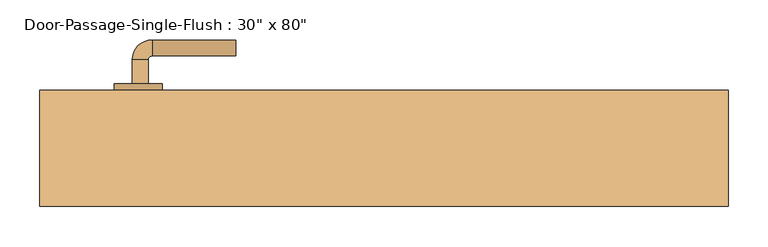
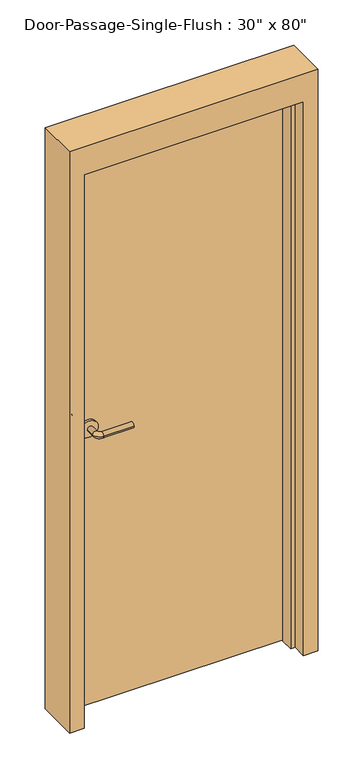
"""IFC4 building model written with IfcOpenShell, lengths in millimetres: door geometry."""

from ifc_helpers import new_model, si_unit, point, frame, frame_2d, origin, origin_with_axes, place, context, project, spatial, polyline, circle_curve, ellipse_curve, trimmed, segment, composite_curve, outline, extrude, faceted_brep, source, transform, mapped, element, save
from ifc_brep_helpers import plane_surface, cylinder_surface, revolved_surface, advanced_brep


def door_bb4af967(model_context):
    return source(origin(), model_context, "Body", "SolidModel", [
        advanced_brep(
        [(-315.990625, 4.7, 1016.0), (-295.990625, 4.7, 1016.0), (-295.990625, -25.3, 1016.0), (-315.990625, -25.3, 1016.0), (-290.990625, -30.3, 1016.0), (-290.990625, -50.3, 1016.0), (-185.990625, -50.3, 1016.0), (-185.990625, -30.3, 1016.0)],
        [
            (0, 1, circle_curve(frame((-305.990625, 4.7, 1016.0), z_axis=(0.0, 1.0, 0.0), x_axis=(1.0, 0.0, 0.0)), 10.0)),
            (1, 0, circle_curve(frame((-305.990625, 4.7, 1016.0), z_axis=(0.0, 1.0, 0.0), x_axis=(1.0, 0.0, 0.0)), 10.0)),
            (1, 2),
            (2, 3, circle_curve(frame((-305.990625, -25.3, 1016.0), z_axis=(0.0, 1.0, 0.0), x_axis=(1.0, 0.0, 0.0)), 10.0)),
            (3, 0),
            (3, 2, circle_curve(frame((-305.990625, -25.3, 1016.0), z_axis=(0.0, 1.0, 0.0), x_axis=(1.0, 0.0, 0.0)), 10.0)),
            (4, 5, circle_curve(frame((-290.990625, -40.3, 1016.0), z_axis=(-1.0, 0.0, 0.0), x_axis=(0.0, 1.0, 0.0)), 10.0)),
            (5, 3, circle_curve(frame((-290.990625, -25.3, 1016.0), z_axis=(0.0, 0.0, -1.0), x_axis=(-1.0, 0.0, 0.0)), 25.0)),
            (2, 4, circle_curve(frame((-290.990625, -25.3, 1016.0), z_axis=(0.0, 0.0, 1.0), x_axis=(-1.0, 0.0, 0.0)), 5.0)),
            (5, 4, circle_curve(frame((-290.990625, -40.3, 1016.0), z_axis=(-1.0, 0.0, 0.0), x_axis=(0.0, 1.0, 0.0)), 10.0)),
            (6, 7, circle_curve(frame((-185.990625, -40.3, 1016.0), z_axis=(1.0, 0.0, 0.0), x_axis=(0.0, 1.0, 0.0)), 10.0)),
            (7, 6, circle_curve(frame((-185.990625, -40.3, 1016.0), z_axis=(1.0, 0.0, 0.0), x_axis=(0.0, 1.0, 0.0)), 10.0)),
            (4, 7),
            (6, 5),
        ],
        [
            plane_surface(frame((-305.990625, 4.7, 1016.0), z_axis=(0.0, 1.0, 0.0), x_axis=(0.0, 0.0, 1.0))),
            cylinder_surface(frame((-305.990625, 4.7, 1016.0), z_axis=(0.0, 1.0, 0.0), x_axis=(1.0, 0.0, 0.0)), 10.0),
            revolved_surface(trimmed(ellipse_curve(frame((-305.990625, -25.3, 1016.0), z_axis=(0.0, -1.0, 0.0), x_axis=(1.0, 0.0, 0.0)), 10.0, 10.0), [point((-315.990625, -25.3, 1016.0))], [point((-295.990625, -25.3, 1016.0))], True, "CARTESIAN"), (-290.990625, -25.3, 1016.0), (0.0, 0.0, -1.0)),
            revolved_surface(trimmed(ellipse_curve(frame((-305.990625, -25.3, 1016.0), z_axis=(0.0, -1.0, 0.0), x_axis=(1.0, 0.0, 0.0)), 10.0, 10.0), [point((-295.990625, -25.3, 1016.0))], [point((-315.990625, -25.3, 1016.0))], True, "CARTESIAN"), (-290.990625, -25.3, 1016.0), (0.0, 0.0, -1.0)),
            plane_surface(frame((-185.990625, -40.3, 1016.0), z_axis=(1.0, 0.0, 0.0), x_axis=(0.0, 0.0, 1.0))),
            cylinder_surface(frame((-290.990625, -40.3, 1016.0), z_axis=(-1.0, 0.0, 0.0), x_axis=(0.0, 1.0, 0.0)), 10.0),
        ],
        [
            (0, [[1, 2]]),
            (1, [[3, 4, 5, -2]]),
            (1, [[-5, 6, -3, -1]]),
            (2, [[7, 8, -4, 9]]),
            (3, [[10, -9, -6, -8]]),
            (4, [[11, 12]]),
            (5, [[13, -11, 14, -7]]),
            (5, [[-14, -12, -13, -10]]),
        ],
    ),
        extrude(outline(composite_curve([segment(trimmed(circle_curve(frame_2d((1016.0, -308.490625)), 30.0), [point((1016.0, -338.490625))], [point((1016.0, -278.490625))], False, "CARTESIAN"), True, "CONTINUOUS"), segment(trimmed(circle_curve(frame_2d((1016.0, -308.490625)), 30.0), [point((1016.0, -278.490625))], [point((1016.0, -338.490625))], False, "CARTESIAN"), True, "CONTINUOUS")], self_intersect=False)), frame((0.0, 4.7, 0.0), z_axis=(0.0, 1.0, 0.0), x_axis=(0.0, 0.0, 1.0)), (0.0, 0.0, 1.0), 8.0),
        advanced_brep(
        [(-315.990625, 65.15, 1016.0), (-295.990625, 65.15, 1016.0), (-315.990625, 95.15, 1016.0), (-295.990625, 95.15, 1016.0), (-290.990625, 100.15, 1016.0), (-290.990625, 120.15, 1016.0), (-185.990625, 120.15, 1016.0), (-185.990625, 100.15, 1016.0)],
        [
            (0, 1, circle_curve(frame((-305.990625, 65.15, 1016.0), z_axis=(0.0, -1.0, 0.0), x_axis=(1.0, 0.0, 0.0)), 10.0)),
            (1, 0, circle_curve(frame((-305.990625, 65.15, 1016.0), z_axis=(0.0, -1.0, 0.0), x_axis=(1.0, 0.0, 0.0)), 10.0)),
            (0, 2),
            (2, 3, circle_curve(frame((-305.990625, 95.15, 1016.0), z_axis=(0.0, -1.0, 0.0), x_axis=(1.0, 0.0, 0.0)), 10.0)),
            (3, 1),
            (3, 2, circle_curve(frame((-305.990625, 95.15, 1016.0), z_axis=(0.0, -1.0, 0.0), x_axis=(1.0, 0.0, 0.0)), 10.0)),
            (4, 3, circle_curve(frame((-290.990625, 95.15, 1016.0), z_axis=(0.0, 0.0, 1.0), x_axis=(-1.0, 0.0, 0.0)), 5.0)),
            (2, 5, circle_curve(frame((-290.990625, 95.15, 1016.0), z_axis=(0.0, 0.0, -1.0), x_axis=(-1.0, 0.0, 0.0)), 25.0)),
            (5, 4, circle_curve(frame((-290.990625, 110.15, 1016.0), z_axis=(-1.0, 0.0, 0.0), x_axis=(0.0, -1.0, 0.0)), 10.0)),
            (4, 5, circle_curve(frame((-290.990625, 110.15, 1016.0), z_axis=(-1.0, 0.0, 0.0), x_axis=(0.0, -1.0, 0.0)), 10.0)),
            (6, 7, circle_curve(frame((-185.990625, 110.15, 1016.0), z_axis=(1.0, 0.0, 0.0), x_axis=(0.0, -1.0, 0.0)), 10.0)),
            (7, 6, circle_curve(frame((-185.990625, 110.15, 1016.0), z_axis=(1.0, 0.0, 0.0), x_axis=(0.0, -1.0, 0.0)), 10.0)),
            (5, 6),
            (7, 4),
        ],
        [
            plane_surface(frame((-305.990625, 65.15, 1016.0), z_axis=(0.0, -1.0, 0.0), x_axis=(0.0, 0.0, 1.0))),
            cylinder_surface(frame((-305.990625, 65.15, 1016.0), z_axis=(0.0, -1.0, 0.0), x_axis=(1.0, 0.0, 0.0)), 10.0),
            revolved_surface(trimmed(ellipse_curve(frame((-305.990625, 95.15, 1016.0), z_axis=(0.0, -1.0, 0.0), x_axis=(1.0, 0.0, 0.0)), 10.0, 10.0), [point((-315.990625, 95.15, 1016.0))], [point((-295.990625, 95.15, 1016.0))], True, "CARTESIAN"), (-290.990625, 95.15, 1016.0), (0.0, 0.0, -1.0)),
            revolved_surface(trimmed(ellipse_curve(frame((-305.990625, 95.15, 1016.0), z_axis=(0.0, -1.0, 0.0), x_axis=(1.0, 0.0, 0.0)), 10.0, 10.0), [point((-295.990625, 95.15, 1016.0))], [point((-315.990625, 95.15, 1016.0))], True, "CARTESIAN"), (-290.990625, 95.15, 1016.0), (0.0, 0.0, -1.0)),
            plane_surface(frame((-185.990625, 110.15, 1016.0), z_axis=(1.0, 0.0, 0.0), x_axis=(0.0, 0.0, 1.0))),
            cylinder_surface(frame((-290.990625, 110.15, 1016.0), z_axis=(-1.0, 0.0, 0.0), x_axis=(0.0, -1.0, 0.0)), 10.0),
        ],
        [
            (0, [[1, 2]]),
            (1, [[-1, 3, 4, 5]]),
            (1, [[-2, -5, 6, -3]]),
            (2, [[7, -4, 8, 9]]),
            (3, [[-8, -6, -7, 10]]),
            (4, [[11, 12]]),
            (5, [[-9, 13, -12, 14]]),
            (5, [[-10, -14, -11, -13]]),
        ],
    ),
        extrude(outline(composite_curve([segment(trimmed(circle_curve(frame_2d((1016.0, -308.490625)), 30.0), [point((1016.0, -338.490625))], [point((1016.0, -278.490625))], False, "CARTESIAN"), True, "CONTINUOUS"), segment(trimmed(circle_curve(frame_2d((1016.0, -308.490625)), 30.0), [point((1016.0, -278.490625))], [point((1016.0, -338.490625))], False, "CARTESIAN"), True, "CONTINUOUS")], self_intersect=False)), frame((0.0, 57.15, 0.0), z_axis=(0.0, 1.0, 0.0), x_axis=(0.0, 0.0, 1.0)), (0.0, 0.0, 1.0), 8.0),
        faceted_brep([(381.0, 7.9375, 0.0), (381.0, 57.15, 0.0), (431.8, 57.15, 0.0), (431.8, -88.9, 0.0), (381.0, -88.9, 0.0), (381.0, -39.6875, 0.0), (365.125, -39.6875, 0.0), (365.125, 7.9375, 0.0), (381.0, 7.9375, 2032.0), (381.0, 57.15, 2032.0), (-381.0, 57.15, 2032.0), (-381.0, 57.15, 0.0), (-431.8, 57.15, 0.0), (-431.8, 57.15, 2133.6), (431.8, 57.15, 2133.6), (431.8, -88.9, 2133.6), (-431.8, -88.9, 2133.6), (-431.8, -88.9, 0.0), (-381.0, -88.9, 0.0), (-381.0, -88.9, 2032.0), (381.0, -88.9, 2032.0), (381.0, -39.6875, 2032.0), (-381.0, -39.6875, 2032.0), (-381.0, -39.6875, 0.0), (-365.125, -39.6875, 0.0), (-365.125, -39.6875, 2016.125), (365.125, -39.6875, 2016.125), (365.125, 7.9375, 2016.125), (-365.125, 7.9375, 2016.125), (-365.125, 7.9375, 0.0), (-381.0, 7.9375, 0.0), (-381.0, 7.9375, 2032.0)], [[[0, 1, 2, 3, 4, 5, 6, 7]], [[1, 0, 8, 9]], [[2, 1, 9, 10, 11, 12, 13, 14]], [[3, 2, 14, 15]], [[4, 3, 15, 16, 17, 18, 19, 20]], [[5, 4, 20, 21]], [[6, 5, 21, 22, 23, 24, 25, 26]], [[7, 6, 26, 27]], [[0, 7, 27, 28, 29, 30, 31, 8]], [[9, 8, 31, 10]], [[20, 19, 22, 21]], [[26, 25, 28, 27]], [[12, 11, 30, 29, 24, 23, 18, 17]], [[11, 10, 31, 30]], [[13, 12, 17, 16]], [[19, 18, 23, 22]], [[25, 24, 29, 28]], [[15, 14, 13, 16]]]),
        extrude(outline(polyline([(381.0, 12.7), (-381.0, 12.7), (-381.0, 57.15), (381.0, 57.15), (381.0, 12.7)])), origin_with_axes(), (0.0, 0.0, 1.0), 2032.0),
    ])


if __name__ == "__main__":
    model = new_model("IFC4")
    model_context = context("Model", 3, world=origin())
    ifc_project = project(units=[si_unit("LENGTHUNIT", "METRE", prefix="MILLI")], contexts=[model_context])
    site = spatial("IfcSite", under=ifc_project)
    building = spatial("IfcBuilding", under=site)
    placement = place(None, origin())
    door_shape = door_bb4af967(model_context)
    element("IfcDoor", 1, ObjectType="Door-Passage-Single-Flush : 30\" x 80\"", at=placement, inside=building, context=model_context, shape_type="MappedRepresentation", body=[
        mapped(door_shape, transform((0.0, 0.0, 0.0), x_axis=(1.0, 0.0, 0.0), y_axis=(0.0, 1.0, 0.0), z_axis=(0.0, 0.0, 1.0))),
    ])
    save(model, "model.ifc")

# Revit data of these elements
# Type "Door-Passage-Single-Flush : 30\" x 80\""
#   Type Mark = "10"
#   Assembly Code = "B2030200"
#   Analytic Construction = "Wooden"
#   Thickness = 0' - 1 3/4"
#   Thermal Resistance (R) = 2.5876 (h·ft²·°F)/BTU
#   Swing Angle [instance default] = 90.00°
#   Strike Height = 3' - 4"
#   Rough Width [instance default] = 2' - 10"
#   Rough Height [instance default] = 7' - 0"
#   MF Opening Height [instance default] = 0' - 4"
#   MF Opening Width [instance default] = 0' - 4"
#   Inset Calculate [instance default] = 0' - 4"
#   Masonry Inset [instance default] = 0' - 1"
#   Height = 6' - 8"
#   Width = 2' - 6"
#   Heat Transfer Coefficient (U) = 0.3865 BTU/(h·ft²·°F)
#   Masonry Frame Depth = 0' - 5 3/4"
#   Masonry Frame [instance default] = yes
#   Function = 1
#   Dry Wall Frame [instance default] = no
#   Panel Material = Wood - Birch
#   Frame Material = Metal - Paint Finish - Grey
#   Door Handle Material = Aluminum
#   Visual Light Transmittance = 0
#   Solar Heat Gain Coefficient = 0
#   Wall Closure = (empty or 0)
# Element 1 (IfcDoor, "Door-Passage-Single-Flush : 30\" x 80\"")
#   Materials on its faces: "Aluminum", "Metal - Paint Finish - Grey", "Wood - Birch"
# Materials
#   "Wood - Birch": class "Wood", colour RGB 166 116 52, transparency 0, Cost = 0
#   "Metal - Paint Finish - Grey": class "Paint", colour RGB 104 104 104, transparency 0, Cost = 0
#   "Aluminum": class "Metal", colour RGB 247 247 247, transparency 0, Description = "Aluminum 6061", Cost = 0
